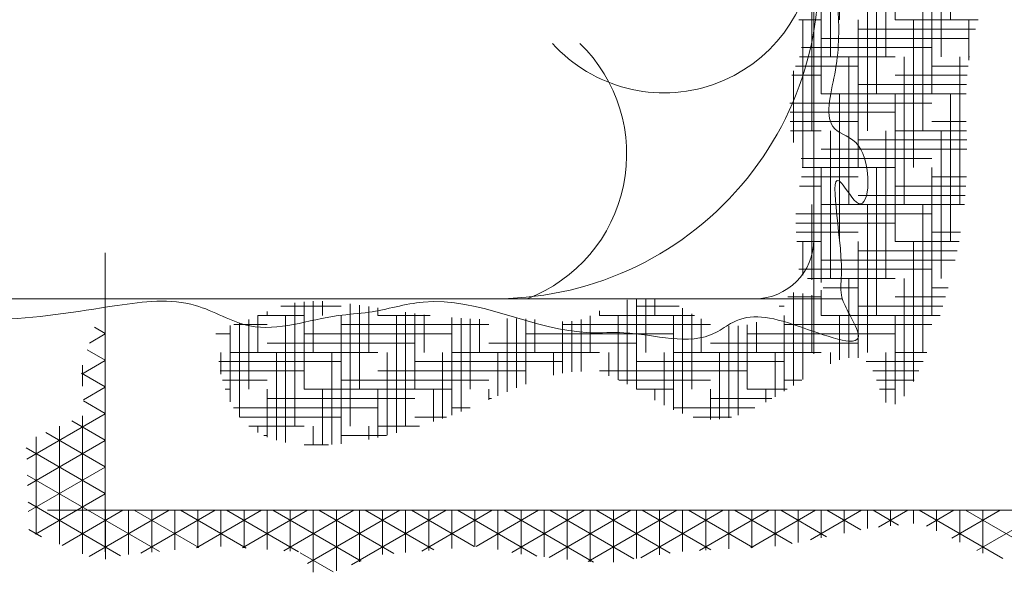
# Model space of a CAD drawing. Units: inches. Extents: x 2330 to 3943, y 1763 to 3461.
# Tile 33 of 40: x 3347 to 3417, y 3025 to 3064. Entities that reach past the tile are written whole.
import ezdxf

# ---------------------------------------------------------------- set-up
doc = ezdxf.new("R2010")
doc.units = ezdxf.units.IN
doc.layers.add('A-FURN', color=8, linetype='Continuous', lineweight=13)

# ---------------------------------------------------------------- blocks, each defined once
blk = doc.blocks.new('A$C200C7901')
for p, q in [((2, 0.2957), (2, 1.2957)), ((1.9974, 0.5977), (1.9974, 0.7977)), ((1.9974, 0.5977), (1.9974, 0.7977)), ((2.0724, 0.5977), (2.0724, 0.7977)), ((2.0724, 0.5977), (2.0724, 0.7977)), ((2.1474, 0.5977), (2.1474, 0.7977)), ((2.1474, 0.5977), (2.1474, 0.7977)), ((1.9849, 0.5477), (1.9849, 0.7477)), ((1.9849, 0.5477), (1.9849, 0.7477)), ((2.0599, 0.5477), (2.0599, 0.7477)), ((2.0599, 0.5477), (2.0599, 0.7477)), ((2.1349, 0.5477), (2.1349, 0.7477)), ((2.1349, 0.5477), (2.1349, 0.7477)), ((1.0407, 0.0275), (1.0407, 0.4323)), ((0.4061, 0.3703), (2.0386, 0.3703)), ((2.4073, 0.0839), (0.9625, 0.0839))]:
    blk.add_line(p, q)
at = {"linetype": 'ByBlock'}
for p, q in [((2.0349, 0.7477), (2.0349, 0.9477)), ((2.0349, 0.7477), (2.0349, 0.9477)), ((2.1099, 0.7477), (2.1099, 0.9477)), ((2.1099, 0.7477), (2.1099, 0.9477)), ((2.1849, 0.7477), (2.1849, 0.9477)), ((2.1849, 0.7477), (2.1849, 0.9477)), ((2.0224, 0.6977), (2.0224, 0.8977)), ((2.0224, 0.6977), (2.0224, 0.8977)), ((2.0974, 0.6977), (2.0974, 0.8977)), ((2.0974, 0.6977), (2.0974, 0.8977)), ((2.1724, 0.6977), (2.1724, 0.8977)), ((2.1724, 0.6977), (2.1724, 0.8977)), ((2.0099, 0.6477), (2.0099, 0.8477)), ((2.0099, 0.6477), (2.0099, 0.8477)), ((2.0849, 0.6477), (2.0849, 0.8477)), ((2.0849, 0.6477), (2.0849, 0.8477)), ((2.1599, 0.6477), (2.1599, 0.8477)), ((2.1599, 0.6477), (2.1599, 0.8477)), ((1.9797, 0.7477), (2.0099, 0.7477)), ((1.9797, 0.7477), (2.0099, 0.7477)), ((2.1099, 0.7477), (2.2222, 0.7477)), ((2.1099, 0.7477), (2.2222, 0.7477)), ((2.2099, 0.6933), (2.2099, 0.7477)), ((2.2099, 0.6933), (2.2099, 0.7477)), ((2.0599, 0.7352), (2.2188, 0.7352)), ((2.0599, 0.7352), (2.2188, 0.7352)), ((2.0099, 0.7227), (2.2099, 0.7227)), ((2.0099, 0.7227), (2.2099, 0.7227)), ((1.9831, 0.7102), (2.1599, 0.7102)), ((1.9831, 0.7102), (2.1599, 0.7102)), ((1.9804, 0.6977), (2.1099, 0.6977)), ((1.9804, 0.6977), (2.1099, 0.6977)), ((2.0474, 0.4977), (2.0474, 0.6977)), ((2.0474, 0.4977), (2.0474, 0.6977)), ((2.1224, 0.4977), (2.1224, 0.6977)), ((2.1224, 0.4977), (2.1224, 0.6977)), ((2.1974, 0.4977), (2.1974, 0.6977)), ((2.1974, 0.4977), (2.1974, 0.6977)), ((2.2099, 0.6977), (2.2106, 0.6977)), ((2.2099, 0.6977), (2.2106, 0.6977)), ((1.9753, 0.6852), (2.0599, 0.6852)), ((1.9753, 0.6852), (2.0599, 0.6852)), ((2.1599, 0.6852), (2.2088, 0.6852)), ((2.1599, 0.6852), (2.2088, 0.6852)), ((1.97, 0.6727), (2.0099, 0.6727)), ((1.97, 0.6727), (2.0099, 0.6727)), ((1.9724, 0.5818), (1.9724, 0.6786)), ((1.9724, 0.5818), (1.9724, 0.6786)), ((2.1099, 0.6727), (2.2075, 0.6727)), ((2.1099, 0.6727), (2.2075, 0.6727)), ((2.0599, 0.6602), (2.2067, 0.6602)), ((2.0599, 0.6602), (2.2067, 0.6602)), ((2.0099, 0.6477), (2.2062, 0.6477)), ((2.0099, 0.6477), (2.2062, 0.6477)), ((2.0349, 0.4477), (2.0349, 0.6477)), ((2.0349, 0.4477), (2.0349, 0.6477)), ((2.1099, 0.4477), (2.1099, 0.6477)), ((2.1099, 0.4477), (2.1099, 0.6477)), ((2.1849, 0.4477), (2.1849, 0.6477)), ((2.1849, 0.4477), (2.1849, 0.6477)), ((1.9673, 0.6352), (2.1599, 0.6352)), ((1.9673, 0.6352), (2.1599, 0.6352)), ((1.9678, 0.6227), (2.1099, 0.6227)), ((1.9678, 0.6227), (2.1099, 0.6227)), ((1.9679, 0.6102), (2.0599, 0.6102)), ((1.9679, 0.6102), (2.0599, 0.6102)), ((2.1599, 0.6102), (2.2064, 0.6102)), ((2.1599, 0.6102), (2.2064, 0.6102)), ((1.9685, 0.5977), (2.0099, 0.5977)), ((1.9685, 0.5977), (2.0099, 0.5977)), ((2.0224, 0.3977), (2.0224, 0.5977)), ((2.0224, 0.3977), (2.0224, 0.5977)), ((2.0974, 0.3977), (2.0974, 0.5977)), ((2.0974, 0.3977), (2.0974, 0.5977)), ((2.1099, 0.5977), (2.2066, 0.5977)), ((2.1099, 0.5977), (2.2066, 0.5977)), ((2.1724, 0.3977), (2.1724, 0.5977)), ((2.1724, 0.3977), (2.1724, 0.5977)), ((2.0599, 0.5852), (2.2069, 0.5852)), ((2.0599, 0.5852), (2.2069, 0.5852)), ((1.9827, 0.5602), (2.1599, 0.5602)), ((1.9827, 0.5602), (2.1599, 0.5602)), ((2.0099, 0.5727), (2.207, 0.5727)), ((2.0099, 0.5727), (2.207, 0.5727)), ((1.9842, 0.5477), (2.1099, 0.5477)), ((1.9842, 0.5477), (2.1099, 0.5477)), ((2.0099, 0.3923), (2.0099, 0.5477)), ((2.0099, 0.3923), (2.0099, 0.5477)), ((2.0849, 0.3477), (2.0849, 0.5477)), ((2.0849, 0.3477), (2.0849, 0.5477)), ((2.1599, 0.3477), (2.1599, 0.5477)), ((2.1599, 0.3477), (2.1599, 0.5477)), ((1.9831, 0.5352), (2.0599, 0.5352)), ((1.9831, 0.5352), (2.0599, 0.5352)), ((2.1599, 0.5352), (2.2065, 0.5352)), ((2.1599, 0.5352), (2.2065, 0.5352)), ((1.9807, 0.5227), (2.0099, 0.5227)), ((1.9807, 0.5227), (2.0099, 0.5227)), ((2.1099, 0.5227), (2.2058, 0.5227)), ((2.1099, 0.5227), (2.2058, 0.5227)), ((2.0599, 0.5102), (2.2049, 0.5102)), ((2.0599, 0.5102), (2.2049, 0.5102)), ((1.9974, 0.3957), (1.9974, 0.4977)), ((1.9974, 0.3957), (1.9974, 0.4977)), ((2.0099, 0.4977), (2.2038, 0.4977)), ((2.0099, 0.4977), (2.2038, 0.4977)), ((2.0724, 0.2977), (2.0724, 0.4977)), ((2.0724, 0.2977), (2.0724, 0.4977)), ((2.1474, 0.2977), (2.1474, 0.4977)), ((2.1474, 0.2977), (2.1474, 0.4977)), ((1.9755, 0.4852), (2.1599, 0.4852)), ((1.9755, 0.4852), (2.1599, 0.4852)), ((1.9757, 0.4727), (2.1099, 0.4727)), ((1.9757, 0.4727), (2.1099, 0.4727)), ((1.9762, 0.4602), (2.0599, 0.4602)), ((1.9762, 0.4602), (2.0599, 0.4602)), ((2.1599, 0.4602), (2.1987, 0.4602)), ((2.1599, 0.4602), (2.1987, 0.4602)), ((1.9768, 0.4477), (2.0099, 0.4477)), ((1.9768, 0.4477), (2.0099, 0.4477)), ((1.9849, 0.402), (1.9849, 0.4477)), ((1.9849, 0.402), (1.9849, 0.4477)), ((2.0599, 0.2903), (2.0599, 0.4477)), ((2.0599, 0.2903), (2.0599, 0.4477)), ((2.1099, 0.4477), (2.1965, 0.4477)), ((2.1099, 0.4477), (2.1965, 0.4477)), ((2.1349, 0.2582), (2.1349, 0.4477)), ((2.1349, 0.2582), (2.1349, 0.4477)), ((2.0599, 0.4352), (2.194, 0.4352)), ((2.0599, 0.4352), (2.194, 0.4352)), ((2.0099, 0.4227), (2.1913, 0.4227)), ((2.0099, 0.4227), (2.1913, 0.4227)), ((1.9797, 0.4102), (2.1599, 0.4102)), ((1.9797, 0.4102), (2.1599, 0.4102)), ((1.9915, 0.3977), (2.1099, 0.3977)), ((1.9915, 0.3977), (2.1099, 0.3977)), ((2.0474, 0.2905), (2.0474, 0.3977)), ((2.0474, 0.2905), (2.0474, 0.3977)), ((2.1224, 0.2385), (2.1224, 0.3977)), ((2.1224, 0.2385), (2.1224, 0.3977)), ((1.9724, 0.253), (1.9724, 0.3785)), ((1.9724, 0.253), (1.9724, 0.3785)), ((1.9849, 0.2609), (1.9849, 0.3774)), ((1.9849, 0.2609), (1.9849, 0.3774)), ((1.9974, 0.2977), (1.9974, 0.3753)), ((1.9974, 0.2977), (1.9974, 0.3753)), ((2.0099, 0.3477), (2.0099, 0.382)), ((2.0099, 0.3477), (2.0099, 0.382)), ((2.0127, 0.3852), (2.0599, 0.3852)), ((2.0127, 0.3852), (2.0599, 0.3852)), ((2.1599, 0.3852), (2.1819, 0.3852)), ((2.1599, 0.3852), (2.1819, 0.3852)), ((1.2785, 0.3602), (1.3599, 0.3602)), ((1.2785, 0.3602), (1.3599, 0.3602)), ((1.2974, 0.1977), (1.2974, 0.3647)), ((1.2974, 0.1977), (1.2974, 0.3647)), ((1.3099, 0.2477), (1.3099, 0.3663)), ((1.3099, 0.2477), (1.3099, 0.3663)), ((1.3224, 0.2977), (1.3224, 0.3669)), ((1.3224, 0.2977), (1.3224, 0.3669)), ((1.3349, 0.3477), (1.3349, 0.3668)), ((1.3349, 0.3477), (1.3349, 0.3668)), ((1.3724, 0.1977), (1.3724, 0.3634)), ((1.3724, 0.1977), (1.3724, 0.3634)), ((1.3849, 0.2477), (1.3849, 0.3616)), ((1.3849, 0.2477), (1.3849, 0.3616)), ((1.7474, 0.2546), (1.7474, 0.3689)), ((1.7474, 0.2546), (1.7474, 0.3689)), ((1.7599, 0.2477), (1.7599, 0.3703)), ((1.7599, 0.2477), (1.7599, 0.3703)), ((1.7599, 0.3602), (1.8177, 0.3602)), ((1.7599, 0.3602), (1.8177, 0.3602)), ((1.7724, 0.2977), (1.7724, 0.3703)), ((1.7724, 0.2977), (1.7724, 0.3703)), ((1.7849, 0.3477), (1.7849, 0.3703)), ((1.7849, 0.3477), (1.7849, 0.3703)), ((1.9532, 0.3602), (1.9599, 0.3602)), ((1.9532, 0.3602), (1.9599, 0.3602)), ((1.9648, 0.3727), (2.0099, 0.3727)), ((1.9648, 0.3727), (2.0099, 0.3727)), ((2.0599, 0.3602), (2.1747, 0.3602)), ((2.0599, 0.3602), (2.1747, 0.3602)), ((2.1099, 0.3727), (2.1784, 0.3727)), ((2.1099, 0.3727), (2.1784, 0.3727)), ((1.2474, 0.2977), (1.2474, 0.3476)), ((1.2474, 0.2977), (1.2474, 0.3476)), ((1.2475, 0.3477), (1.3099, 0.3477)), ((1.2475, 0.3477), (1.3099, 0.3477)), ((1.2599, 0.3477), (1.2599, 0.3531)), ((1.2599, 0.3477), (1.2599, 0.3531)), ((1.2849, 0.1758), (1.2849, 0.3477)), ((1.2849, 0.1758), (1.2849, 0.3477)), ((1.3599, 0.1741), (1.3599, 0.3477)), ((1.3599, 0.1741), (1.3599, 0.3477)), ((1.3974, 0.2977), (1.3974, 0.3597)), ((1.3974, 0.2977), (1.3974, 0.3597)), ((1.4099, 0.3477), (1.4099, 0.3578)), ((1.4099, 0.3477), (1.4099, 0.3578)), ((1.4099, 0.3477), (1.4806, 0.3477)), ((1.4099, 0.3477), (1.4806, 0.3477)), ((1.4349, 0.1886), (1.4349, 0.3477)), ((1.4349, 0.1886), (1.4349, 0.3477)), ((1.4474, 0.1977), (1.4474, 0.3521)), ((1.4474, 0.1977), (1.4474, 0.3521)), ((1.4599, 0.2477), (1.4599, 0.3504)), ((1.4599, 0.2477), (1.4599, 0.3504)), ((1.4724, 0.2977), (1.4724, 0.3487)), ((1.4724, 0.2977), (1.4724, 0.3487)), ((1.6974, 0.2977), (1.6974, 0.3472)), ((1.6974, 0.2977), (1.6974, 0.3472)), ((1.7099, 0.3477), (1.7099, 0.3539)), ((1.7099, 0.3477), (1.7099, 0.3539)), ((1.7099, 0.3477), (1.8383, 0.3477)), ((1.7099, 0.3477), (1.8383, 0.3477)), ((1.7349, 0.2607), (1.7349, 0.3477)), ((1.7349, 0.2607), (1.7349, 0.3477)), ((1.8099, 0.2201), (1.8099, 0.3477)), ((1.8099, 0.2201), (1.8099, 0.3477)), ((1.8224, 0.2148), (1.8224, 0.3575)), ((1.8224, 0.2148), (1.8224, 0.3575)), ((1.8349, 0.2477), (1.8349, 0.3497)), ((1.8349, 0.2477), (1.8349, 0.3497)), ((1.9599, 0.2452), (1.9599, 0.3477)), ((1.9599, 0.2452), (1.9599, 0.3477)), ((2.0099, 0.3477), (2.1708, 0.3477)), ((2.0099, 0.3477), (2.1708, 0.3477)), ((2.0349, 0.2874), (2.0349, 0.3477)), ((2.0349, 0.2874), (2.0349, 0.3477)), ((2.1099, 0.2274), (2.1099, 0.3477)), ((2.1099, 0.2274), (2.1099, 0.3477)), ((1.2099, 0.2308), (1.2099, 0.334)), ((1.2099, 0.2308), (1.2099, 0.334)), ((1.2148, 0.3352), (1.2599, 0.3352)), ((1.2148, 0.3352), (1.2599, 0.3352)), ((1.2224, 0.2106), (1.2224, 0.3375)), ((1.2224, 0.2106), (1.2224, 0.3375)), ((1.2349, 0.2477), (1.2349, 0.3422)), ((1.2349, 0.2477), (1.2349, 0.3422)), ((1.3599, 0.3352), (1.5599, 0.3352)), ((1.3599, 0.3352), (1.5599, 0.3352)), ((1.5099, 0.2129), (1.5099, 0.3447)), ((1.5099, 0.2129), (1.5099, 0.3447)), ((1.5224, 0.2177), (1.5224, 0.3438)), ((1.5224, 0.2177), (1.5224, 0.3438)), ((1.5349, 0.2477), (1.5349, 0.3431)), ((1.5349, 0.2477), (1.5349, 0.3431)), ((1.5474, 0.2977), (1.5474, 0.3428)), ((1.5474, 0.2977), (1.5474, 0.3428)), ((1.5849, 0.2443), (1.5849, 0.3434)), ((1.5849, 0.2443), (1.5849, 0.3434)), ((1.5974, 0.2496), (1.5974, 0.3435)), ((1.5974, 0.2496), (1.5974, 0.3435)), ((1.6099, 0.2546), (1.6099, 0.3432)), ((1.6099, 0.2546), (1.6099, 0.3432)), ((1.6224, 0.2977), (1.6224, 0.3424)), ((1.6224, 0.2977), (1.6224, 0.3424)), ((1.6599, 0.2695), (1.6599, 0.3394)), ((1.6599, 0.2695), (1.6599, 0.3394)), ((1.6599, 0.3352), (1.8599, 0.3352)), ((1.6599, 0.3352), (1.8599, 0.3352)), ((1.6724, 0.2713), (1.6724, 0.3398)), ((1.6724, 0.2713), (1.6724, 0.3398)), ((1.6849, 0.272), (1.6849, 0.3422)), ((1.6849, 0.272), (1.6849, 0.3422)), ((1.8474, 0.2977), (1.8474, 0.3432)), ((1.8474, 0.2977), (1.8474, 0.3432)), ((1.8849, 0.2093), (1.8849, 0.3337)), ((1.8849, 0.2093), (1.8849, 0.3337)), ((1.8974, 0.2129), (1.8974, 0.3335)), ((1.8974, 0.2129), (1.8974, 0.3335)), ((1.9099, 0.2477), (1.9099, 0.3349)), ((1.9099, 0.2477), (1.9099, 0.3349)), ((1.9224, 0.2977), (1.9224, 0.3385)), ((1.9224, 0.2977), (1.9224, 0.3385)), ((1.9599, 0.3352), (2.1599, 0.3352)), ((1.9599, 0.3352), (2.1599, 0.3352)), ((1.0194, 0.3103), (1.0407, 0.3227)), ((1.0194, 0.3103), (1.0407, 0.3227)), ((1.0261, 0.3316), (1.0407, 0.3232)), ((1.0261, 0.3316), (1.0407, 0.3232)), ((1.1904, 0.3227), (1.2099, 0.3227)), ((1.1904, 0.3227), (1.2099, 0.3227)), ((1.3099, 0.3227), (1.5099, 0.3227)), ((1.3099, 0.3227), (1.5099, 0.3227)), ((1.6099, 0.3227), (1.8099, 0.3227)), ((1.6099, 0.3227), (1.8099, 0.3227)), ((1.9099, 0.3227), (2.1099, 0.3227)), ((1.9099, 0.3227), (2.1099, 0.3227)), ((1.2599, 0.3102), (1.4599, 0.3102)), ((1.2599, 0.3102), (1.4599, 0.3102)), ((1.5599, 0.3102), (1.7599, 0.3102)), ((1.5599, 0.3102), (1.7599, 0.3102)), ((1.8599, 0.3102), (2.0599, 0.3102)), ((1.8599, 0.3102), (2.0599, 0.3102)), ((1.0164, 0.3011), (1.0407, 0.2871)), ((1.0164, 0.3011), (1.0407, 0.2871)), ((1.1974, 0.2683), (1.1974, 0.2977)), ((1.1974, 0.2683), (1.1974, 0.2977)), ((1.2099, 0.2977), (1.4099, 0.2977)), ((1.2099, 0.2977), (1.4099, 0.2977)), ((1.2724, 0.1788), (1.2724, 0.2977)), ((1.2724, 0.1788), (1.2724, 0.2977)), ((1.3474, 0.173), (1.3474, 0.2977)), ((1.3474, 0.173), (1.3474, 0.2977)), ((1.4224, 0.1854), (1.4224, 0.2977)), ((1.4224, 0.1854), (1.4224, 0.2977)), ((1.4974, 0.2083), (1.4974, 0.2977)), ((1.4974, 0.2083), (1.4974, 0.2977)), ((1.5099, 0.2977), (1.7099, 0.2977)), ((1.5099, 0.2977), (1.7099, 0.2977)), ((1.5724, 0.2389), (1.5724, 0.2977)), ((1.5724, 0.2389), (1.5724, 0.2977)), ((1.6474, 0.2668), (1.6474, 0.2977)), ((1.6474, 0.2668), (1.6474, 0.2977)), ((1.7224, 0.2658), (1.7224, 0.2977)), ((1.7224, 0.2658), (1.7224, 0.2977)), ((1.7974, 0.2263), (1.7974, 0.2977)), ((1.7974, 0.2263), (1.7974, 0.2977)), ((1.8099, 0.2977), (2.0099, 0.2977)), ((1.8099, 0.2977), (2.0099, 0.2977)), ((1.8724, 0.2072), (1.8724, 0.2977)), ((1.8724, 0.2072), (1.8724, 0.2977)), ((1.9474, 0.2376), (1.9474, 0.2977)), ((1.9474, 0.2376), (1.9474, 0.2977)), ((2.0224, 0.2822), (2.0224, 0.2977)), ((2.0224, 0.2822), (2.0224, 0.2977)), ((2.0974, 0.2299), (2.0974, 0.2977)), ((2.0974, 0.2299), (2.0974, 0.2977)), ((2.1099, 0.2977), (2.153, 0.2977)), ((2.1099, 0.2977), (2.153, 0.2977)), ((1.0089, 0.2682), (1.0407, 0.2866)), ((1.0089, 0.2682), (1.0407, 0.2866)), ((1.0099, 0.2521), (1.0099, 0.2804)), ((1.0099, 0.2521), (1.0099, 0.2804)), ((1.1943, 0.2852), (1.3599, 0.2852)), ((1.1943, 0.2852), (1.3599, 0.2852)), ((1.4599, 0.2852), (1.6599, 0.2852)), ((1.4599, 0.2852), (1.6599, 0.2852)), ((1.7599, 0.2852), (1.9599, 0.2852)), ((1.7599, 0.2852), (1.9599, 0.2852)), ((2.0708, 0.2852), (2.1478, 0.2852)), ((2.0708, 0.2852), (2.1478, 0.2852)), ((1.0088, 0.2694), (1.0407, 0.251)), ((1.0088, 0.2694), (1.0407, 0.251)), ((1.1965, 0.2727), (1.3099, 0.2727)), ((1.1965, 0.2727), (1.3099, 0.2727)), ((1.4099, 0.2727), (1.6099, 0.2727)), ((1.4099, 0.2727), (1.6099, 0.2727)), ((1.7099, 0.2727), (1.9099, 0.2727)), ((1.7099, 0.2727), (1.9099, 0.2727)), ((2.08, 0.2727), (2.1422, 0.2727)), ((2.08, 0.2727), (2.1422, 0.2727)), ((1.1994, 0.2602), (1.2599, 0.2602)), ((1.1994, 0.2602), (1.2599, 0.2602)), ((1.3599, 0.2602), (1.5599, 0.2602)), ((1.3599, 0.2602), (1.5599, 0.2602)), ((1.7361, 0.2602), (1.8599, 0.2602)), ((1.7361, 0.2602), (1.8599, 0.2602)), ((1.9599, 0.2602), (1.9838, 0.2602)), ((1.9599, 0.2602), (1.9838, 0.2602)), ((2.0848, 0.2602), (2.1359, 0.2602)), ((2.0848, 0.2602), (2.1359, 0.2602)), ((1.0111, 0.2334), (1.0407, 0.2505)), ((1.0111, 0.2334), (1.0407, 0.2505)), ((1.2031, 0.2477), (1.2099, 0.2477)), ((1.2031, 0.2477), (1.2099, 0.2477)), ((1.2599, 0.1831), (1.2599, 0.2477)), ((1.2599, 0.1831), (1.2599, 0.2477)), ((1.3099, 0.2477), (1.5099, 0.2477)), ((1.3099, 0.2477), (1.5099, 0.2477)), ((1.3349, 0.1723), (1.3349, 0.2477)), ((1.3349, 0.1723), (1.3349, 0.2477)), ((1.4099, 0.1825), (1.4099, 0.2477)), ((1.4099, 0.1825), (1.4099, 0.2477)), ((1.4849, 0.2039), (1.4849, 0.2477)), ((1.4849, 0.2039), (1.4849, 0.2477)), ((1.5599, 0.2335), (1.5599, 0.2477)), ((1.5599, 0.2335), (1.5599, 0.2477)), ((1.7599, 0.2477), (1.8099, 0.2477)), ((1.7599, 0.2477), (1.8099, 0.2477)), ((1.7849, 0.2332), (1.7849, 0.2477)), ((1.7849, 0.2332), (1.7849, 0.2477)), ((1.8599, 0.2068), (1.8599, 0.2477)), ((1.8599, 0.2068), (1.8599, 0.2477)), ((1.9099, 0.2477), (1.9639, 0.2477)), ((1.9099, 0.2477), (1.9639, 0.2477)), ((1.9349, 0.2304), (1.9349, 0.2477)), ((1.9349, 0.2304), (1.9349, 0.2477)), ((2.0888, 0.2477), (2.1099, 0.2477)), ((2.0888, 0.2477), (2.1099, 0.2477)), ((1.0112, 0.232), (1.0407, 0.215)), ((1.0112, 0.232), (1.0407, 0.215)), ((1.2599, 0.2352), (1.4599, 0.2352)), ((1.2599, 0.2352), (1.4599, 0.2352)), ((1.5599, 0.2352), (1.5638, 0.2352)), ((1.5599, 0.2352), (1.5638, 0.2352)), ((1.8599, 0.2352), (1.9433, 0.2352)), ((1.8599, 0.2352), (1.9433, 0.2352)), ((0.9344, 0.153), (1.0407, 0.2144)), ((0.9344, 0.153), (1.0407, 0.2144)), ((1.2142, 0.2227), (1.4099, 0.2227)), ((1.2142, 0.2227), (1.4099, 0.2227)), ((1.5099, 0.2227), (1.5346, 0.2227)), ((1.5099, 0.2227), (1.5346, 0.2227)), ((1.8099, 0.2227), (1.9203, 0.2227)), ((1.8099, 0.2227), (1.9203, 0.2227)), ((0.9953, 0.2051), (1.0407, 0.1789)), ((0.9953, 0.2051), (1.0407, 0.1789)), ((1.0099, 0.0251), (1.0099, 0.2117)), ((1.0099, 0.0251), (1.0099, 0.2117)), ((1.2227, 0.2102), (1.3599, 0.2102)), ((1.2227, 0.2102), (1.3599, 0.2102)), ((1.4599, 0.2102), (1.5027, 0.2102)), ((1.4599, 0.2102), (1.5027, 0.2102)), ((1.8368, 0.2102), (1.8884, 0.2102)), ((1.8368, 0.2102), (1.8884, 0.2102)), ((0.9602, 0.1893), (1.0407, 0.1428)), ((0.9602, 0.1893), (1.0407, 0.1428)), ((0.9787, 0.0381), (0.9787, 0.1976)), ((0.9787, 0.0381), (0.9787, 0.1976)), ((1.2351, 0.1977), (1.3099, 0.1977)), ((1.2351, 0.1977), (1.3099, 0.1977)), ((1.2474, 0.1892), (1.2474, 0.1977)), ((1.2474, 0.1892), (1.2474, 0.1977)), ((1.3224, 0.1722), (1.3224, 0.1977)), ((1.3224, 0.1722), (1.3224, 0.1977)), ((1.3974, 0.1799), (1.3974, 0.1977)), ((1.3974, 0.1799), (1.3974, 0.1977)), ((1.4099, 0.1977), (1.4662, 0.1977)), ((1.4099, 0.1977), (1.4662, 0.1977)), ((0.9355, 0.1176), (1.0407, 0.1783)), ((0.9355, 0.1176), (1.0407, 0.1783)), ((0.9474, 0.0512), (0.9474, 0.1835)), ((0.9474, 0.0512), (0.9474, 0.1835)), ((1.2552, 0.1852), (1.2599, 0.1852)), ((1.2552, 0.1852), (1.2599, 0.1852)), ((1.3599, 0.1852), (1.4215, 0.1852)), ((1.3599, 0.1852), (1.4215, 0.1852)), ((0.9339, 0.1684), (1.0407, 0.1067)), ((0.9339, 0.1684), (1.0407, 0.1067)), ((1.3099, 0.1727), (1.3428, 0.1727)), ((1.3099, 0.1727), (1.3428, 0.1727)), ((0.9366, 0.0822), (1.0407, 0.1422)), ((0.9366, 0.0822), (1.0407, 0.1422)), ((2.2208, 0.0297), (2.4078, 0.1377)), ((2.2208, 0.0297), (2.4078, 0.1377)), ((0.935, 0.1316), (1.114, 0.0283)), ((0.935, 0.1316), (1.114, 0.0283)), ((0.9362, 0.0948), (1.0616, 0.0225)), ((0.9362, 0.0948), (1.0616, 0.0225)), ((0.9463, 0.0516), (1.0407, 0.1061)), ((0.9463, 0.0516), (1.0407, 0.1061)), ((0.9826, 0.0365), (1.0647, 0.0839)), ((0.9826, 0.0365), (1.0647, 0.0839)), ((1.0189, 0.0214), (1.1272, 0.0839)), ((1.0189, 0.0214), (1.1272, 0.0839)), ((1.0412, 0.0179), (1.0412, 0.0839)), ((1.0412, 0.0179), (1.0412, 0.0839)), ((1.0724, 0.0243), (1.0724, 0.0839)), ((1.0724, 0.0243), (1.0724, 0.0839)), ((1.0801, 0.0839), (1.1675, 0.0335)), ((1.0801, 0.0839), (1.1675, 0.0335)), ((1.0891, 0.0259), (1.1897, 0.0839)), ((1.0891, 0.0259), (1.1897, 0.0839)), ((1.1037, 0.0273), (1.1037, 0.0839)), ((1.1037, 0.0273), (1.1037, 0.0839)), ((1.1349, 0.0303), (1.1349, 0.0839)), ((1.1349, 0.0303), (1.1349, 0.0839)), ((1.1426, 0.0839), (1.2313, 0.0327)), ((1.1426, 0.0839), (1.2313, 0.0327)), ((1.1642, 0.0331), (1.2522, 0.0839)), ((1.1642, 0.0331), (1.2522, 0.0839)), ((1.1662, 0.0333), (1.1662, 0.0839)), ((1.1662, 0.0333), (1.1662, 0.0839)), ((1.1974, 0.0351), (1.1974, 0.0839)), ((1.1974, 0.0351), (1.1974, 0.0839)), ((1.2051, 0.0839), (1.3023, 0.0278)), ((1.2051, 0.0839), (1.3023, 0.0278)), ((1.2266, 0.033), (1.3147, 0.0839)), ((1.2266, 0.033), (1.3147, 0.0839)), ((1.2287, 0.0329), (1.2287, 0.0839)), ((1.2287, 0.0329), (1.2287, 0.0839)), ((1.2599, 0.0308), (1.2599, 0.0839)), ((1.2599, 0.0308), (1.2599, 0.0839)), ((1.2676, 0.0839), (1.3871, 0.015)), ((1.2676, 0.0839), (1.3871, 0.015)), ((1.2824, 0.0292), (1.3772, 0.0839)), ((1.2824, 0.0292), (1.3772, 0.0839)), ((1.2912, 0.0286), (1.2912, 0.0839)), ((1.2912, 0.0286), (1.2912, 0.0839)), ((1.3146, 0.0117), (1.4397, 0.0839)), ((1.3146, 0.0117), (1.4397, 0.0839)), ((1.3224, 0), (1.3224, 0.0839)), ((1.3224, 0), (1.3224, 0.0839)), ((1.3301, 0.0839), (1.4312, 0.0256)), ((1.3301, 0.0839), (1.4312, 0.0256)), ((1.3537, 0.0022), (1.3537, 0.0839)), ((1.3537, 0.0022), (1.3537, 0.0839)), ((1.3743, 0.0101), (1.5022, 0.0839)), ((1.3743, 0.0101), (1.5022, 0.0839)), ((1.3849, 0.0141), (1.3849, 0.0839)), ((1.3849, 0.0141), (1.3849, 0.0839)), ((1.3926, 0.0839), (1.4856, 0.0302)), ((1.3926, 0.0839), (1.4856, 0.0302)), ((1.4162, 0.0243), (1.4162, 0.0839)), ((1.4162, 0.0243), (1.4162, 0.0839)), ((1.4474, 0.027), (1.4474, 0.0839)), ((1.4474, 0.027), (1.4474, 0.0839)), ((1.4551, 0.0839), (1.54, 0.0349)), ((1.4551, 0.0839), (1.54, 0.0349)), ((1.4693, 0.0288), (1.5647, 0.0839)), ((1.4693, 0.0288), (1.5647, 0.0839)), ((1.4787, 0.0296), (1.4787, 0.0839)), ((1.4787, 0.0296), (1.4787, 0.0839)), ((1.5099, 0.0323), (1.5099, 0.0839)), ((1.5099, 0.0323), (1.5099, 0.0839)), ((1.5176, 0.0839), (1.6251, 0.0219)), ((1.5176, 0.0839), (1.6251, 0.0219)), ((1.5412, 0.035), (1.5412, 0.0839)), ((1.5412, 0.035), (1.5412, 0.0839)), ((1.5427, 0.0351), (1.6272, 0.0839)), ((1.5427, 0.0351), (1.6272, 0.0839)), ((1.5724, 0.0308), (1.5724, 0.0839)), ((1.5724, 0.0308), (1.5724, 0.0839)), ((1.5801, 0.0839), (1.7018, 0.0137)), ((1.5801, 0.0839), (1.7018, 0.0137)), ((1.5911, 0.027), (1.6897, 0.0839)), ((1.5911, 0.027), (1.6897, 0.0839)), ((1.6037, 0.0245), (1.6037, 0.0839)), ((1.6037, 0.0245), (1.6037, 0.0839)), ((1.6349, 0.0208), (1.6349, 0.0839)), ((1.6349, 0.0208), (1.6349, 0.0839)), ((1.6416, 0.0201), (1.7522, 0.0839)), ((1.6416, 0.0201), (1.7522, 0.0839)), ((1.6426, 0.0839), (1.7565, 0.0182)), ((1.6426, 0.0839), (1.7565, 0.0182)), ((1.6662, 0.0175), (1.6662, 0.0839)), ((1.6662, 0.0175), (1.6662, 0.0839)), ((1.6944, 0.0145), (1.8147, 0.0839)), ((1.6944, 0.0145), (1.8147, 0.0839)), ((1.6974, 0.0141), (1.6974, 0.0839)), ((1.6974, 0.0141), (1.6974, 0.0839)), ((1.7051, 0.0839), (1.8054, 0.026)), ((1.7051, 0.0839), (1.8054, 0.026)), ((1.7287, 0.0137), (1.7287, 0.0839)), ((1.7287, 0.0137), (1.7287, 0.0839)), ((1.7599, 0.0187), (1.7599, 0.0839)), ((1.7599, 0.0187), (1.7599, 0.0839)), ((1.7659, 0.0197), (1.8772, 0.0839)), ((1.7659, 0.0197), (1.8772, 0.0839)), ((1.7676, 0.0839), (1.8606, 0.0303)), ((1.7676, 0.0839), (1.8606, 0.0303)), ((1.7912, 0.0237), (1.7912, 0.0839)), ((1.7912, 0.0237), (1.7912, 0.0839)), ((1.8224, 0.0281), (1.8224, 0.0839)), ((1.8224, 0.0281), (1.8224, 0.0839)), ((1.8301, 0.0839), (1.9175, 0.0335)), ((1.8301, 0.0839), (1.9175, 0.0335)), ((1.8452, 0.0294), (1.9397, 0.0839)), ((1.8452, 0.0294), (1.9397, 0.0839)), ((1.8537, 0.0299), (1.8537, 0.0839)), ((1.8537, 0.0299), (1.8537, 0.0839)), ((1.8849, 0.0316), (1.8849, 0.0839)), ((1.8849, 0.0316), (1.8849, 0.0839)), ((1.8926, 0.0839), (1.9706, 0.0389)), ((1.8926, 0.0839), (1.9706, 0.0389)), ((1.9146, 0.0333), (2.0022, 0.0839)), ((1.9146, 0.0333), (2.0022, 0.0839)), ((1.9162, 0.0334), (1.9162, 0.0839)), ((1.9162, 0.0334), (1.9162, 0.0839)), ((1.9474, 0.0352), (1.9474, 0.0839)), ((1.9474, 0.0352), (1.9474, 0.0839)), ((1.9551, 0.0839), (2.017, 0.0482)), ((1.9551, 0.0839), (2.017, 0.0482)), ((1.9787, 0.0405), (1.9787, 0.0839)), ((1.9787, 0.0405), (1.9787, 0.0839)), ((1.9953, 0.0438), (2.0647, 0.0839)), ((1.9953, 0.0438), (2.0647, 0.0839)), ((2.0099, 0.0468), (2.0099, 0.0839)), ((2.0099, 0.0468), (2.0099, 0.0839)), ((2.0176, 0.0839), (2.0634, 0.0575)), ((2.0176, 0.0839), (2.0634, 0.0575)), ((2.0412, 0.053), (2.0412, 0.0839)), ((2.0412, 0.053), (2.0412, 0.0839)), ((2.0724, 0.0592), (2.0724, 0.0839)), ((2.0724, 0.0592), (2.0724, 0.0839)), ((2.0801, 0.0839), (2.1147, 0.0639)), ((2.0801, 0.0839), (2.1147, 0.0639)), ((2.0873, 0.0609), (2.1272, 0.0839)), ((2.0873, 0.0609), (2.1272, 0.0839)), ((2.1037, 0.0627), (2.1037, 0.0839)), ((2.1037, 0.0627), (2.1037, 0.0839)), ((2.1349, 0.0662), (2.1349, 0.0839)), ((2.1349, 0.0662), (2.1349, 0.0839)), ((2.1426, 0.0839), (2.2557, 0.0186)), ((2.1426, 0.0839), (2.2557, 0.0186)), ((2.1526, 0.0625), (2.1897, 0.0839)), ((2.1526, 0.0625), (2.1897, 0.0839)), ((2.1662, 0.056), (2.1662, 0.0839)), ((2.1662, 0.056), (2.1662, 0.0839)), ((2.1867, 0.0461), (2.2522, 0.0839)), ((2.1867, 0.0461), (2.2522, 0.0839)), ((2.1974, 0.041), (2.1974, 0.0839)), ((2.1974, 0.041), (2.1974, 0.0839)), ((2.2051, 0.0839), (2.2913, 0.0342)), ((2.2051, 0.0839), (2.2913, 0.0342)), ((2.2287, 0.0259), (2.2287, 0.0839)), ((2.2287, 0.0259), (2.2287, 0.0839)), ((0.9374, 0.0581), (0.9545, 0.0482)), ((0.9374, 0.0581), (0.9545, 0.0482)), ((1.3048, 0.0264), (1.3494, 0.0006)), ((1.3048, 0.0264), (1.3494, 0.0006))]:
    blk.add_line(p, q, dxfattribs=at)
for centre, radius, start, end in [((1.5693, 0.8075), 0.4372, 269.0679, 9.9322), ((1.7969, 0.8525), 0.2035, 222.1514, 356.4639), ((1.5372, 0.5659), 0.2094, 290.9415, 45.7647), ((1.92, 0.4503), 0.08, 270, 0)]:
    blk.add_arc(centre, radius, start, end)
blk.add_open_spline([(0.473, 1.2954), (0.4739, 1.2781), (0.4755, 1.2477), (0.5032, 1.2084), (0.4801, 1.1701), (0.4928, 1.1255), (0.4674, 1.0912), (0.4579, 1.0351), (0.501, 0.9724), (0.4311, 0.8832), (0.4902, 0.8637), (0.4843, 0.8288), (0.4774, 0.7906), (0.4625, 0.7457), (0.459, 0.6999), (0.4816, 0.6664), (0.4748, 0.625), (0.4791, 0.5889), (0.4533, 0.5528), (0.4738, 0.5004), (0.4658, 0.4502), (0.4696, 0.3946), (0.4189, 0.3935), (0.4493, 0.3684), (0.4694, 0.3857), (0.4922, 0.3576), (0.5297, 0.3262), (0.5917, 0.3353), (0.6454, 0.3754), (0.7083, 0.3741), (0.7643, 0.3328), (0.826, 0.346), (0.925, 0.3388), (1.0353, 0.3593), (1.1561, 0.3744), (1.2477, 0.3154), (1.3302, 0.3474), (1.4086, 0.3512), (1.5217, 0.3878), (1.6362, 0.3176), (1.7682, 0.3285), (1.8402, 0.3019), (1.9071, 0.3529), (1.9647, 0.3412), (2.0795, 0.2948), (2.0472, 0.3498), (2.0343, 0.3772), (2.0435, 0.43), (2.0109, 0.5782), (2.0746, 0.4643), (2.0805, 0.584), (2.0084, 0.5979), (2.0343, 0.6846), (2.0344, 0.746), (2.0293, 0.8096), (2.0489, 0.8545), (2.0652, 0.9218), (1.9842, 0.9297), (2.0007, 1.0162), (2.0367, 1.0585), (2.0367, 1.1102), (2.0457, 1.1647), (2.0226, 1.2084), (2.0234, 1.2306), (2.0236, 1.2352)], degree=3, knots=[0, 0, 0, 0, 51.660678, 90.967412, 128.902454, 170.303599, 219.852997, 247.834962, 336.321557, 429.35469, 458.821847, 477.222321, 524.135809, 581.038434, 617.839381, 657.146115, 693.947125, 740.178081, 760.753248, 820.731705, 885.133458, 928.777044, 953.563729, 976.574207, 995.553042, 1018.563482, 1064.584401, 1147.951297, 1174.787598, 1266.851571, 1308.018447, 1377.066427, 1441.511314, 1608.245014, 1714.11869, 1792.771707, 1913.247991, 1954.931389, 2029.864445, 2259.189419, 2305.221512, 2429.507982, 2456.344283, 2543.92595, 2627.925037, 2662.96218, 2687.736879, 2719.937755, 2839.540991, 2875.47895, 2953.681041, 2993.270313, 3066.872333, 3154.395764, 3200.397042, 3248.426375, 3312.828127, 3347.881398, 3444.484026, 3481.577522, 3518.665244, 3592.267265, 3644.719162, 3658.519501, 3658.519501, 3658.519501, 3658.519501], dxfattribs=at)

msp = doc.modelspace()

# ---------------------------------------------------------------- block references
at = {"layer": 'A-FURN', "xscale": 52.5181391560459, "yscale": 52.5181391560459, "zscale": 52.5181391560459}
msp.add_blockref('A$C200C7901', (3298.7219, 3025.0763), dxfattribs=at)

doc.saveas('drawing.dxf')
